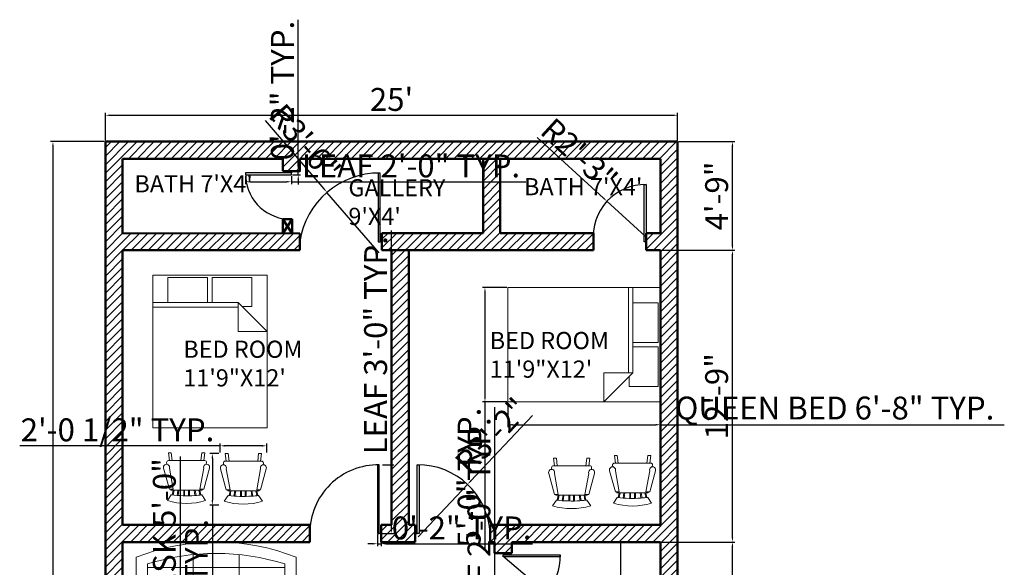
# Model space of a CAD drawing. Units: inches. Extents: x 2308 to 2824, y 1390 to 2024.
# Tile 2 of 2: x 2308 to 2824, y 1737 to 2024. Entities that reach past the tile are written whole.
import ezdxf

# ---------------------------------------------------------------- set-up
doc = ezdxf.new("R2010")
doc.units = ezdxf.units.IN
for name, color, linetype, lineweight in [('A-ANNO-DIMS', 2, 'Continuous', 18), ('A-DOOR', 4, 'Continuous', 25), ('A-FLOR-FIXT', 9, 'Continuous', 25), ('A-FURN', 8, 'Continuous', 18), ('A-WALL', 7, 'Continuous', 50)]:
    doc.layers.add(name, color=color, linetype=linetype, lineweight=lineweight)
doc.layers.add('A-AREA-IDEN', color=244, linetype='Continuous', lineweight=25, true_color=0x991b1e)
doc.layers.add('A-WALL-PATT', color=177, linetype='Continuous', lineweight=13, true_color=0x293189)
doc.styles.get("Standard").update_dxf_attribs({"font": 'arial.ttf'})
doc.dimstyles.new('ISO-25', dxfattribs={"dimtxt": 12, "dimasz": 2.5, "dimexe": 1.25, "dimexo": 0.625, "dimtad": 1, "dimdec": 1, "dimlunit": 3, "dimtxsty": 'Standard', "dimcen": 2.5, "dimadec": 0, "dimazin": 0, "dimtfac": 1, "dimtdec": 1, "dimtmove": 0, "dimatfit": 3, "dimfxl": 1, "dimarcsym": 0})

# ---------------------------------------------------------------- blocks, each defined once
blk = doc.blocks.new('*D1')
at = {"layer": 'A-ANNO-DIMS', "color": 0, "lineweight": -2, "transparency": 16777216}
for p, q in [((2352.46, 1961.09), (2352.46, 1975.53)), ((2354.96, 1974.28), (2649.96, 1974.28)), ((2652.46, 1961.09), (2652.46, 1975.53))]:
    blk.add_line(p, q, dxfattribs=at)
at = {"layer": 'A-ANNO-DIMS', "color": 0, "transparency": 16777216}
for points in [[(2354.96, 1974.7), (2354.96, 1973.86), (2352.46, 1974.28)], [(2649.96, 1974.7), (2649.96, 1973.86), (2652.46, 1974.28)]]:
    blk.add_solid(points, dxfattribs=at)
at = {"layer": 'Defpoints', "color": 0, "transparency": 16777216}
for p in [(2652.46, 1974.28), (2352.46, 1960.47), (2652.46, 1960.47)]:
    blk.add_point(p, dxfattribs=at)
at = {"layer": 'A-ANNO-DIMS', "color": 0, "transparency": 16777216, "insert": (2502.46, 1981.03), "char_height": 12, "attachment_point": 5}
blk.add_mtext("25'", dxfattribs=at)
blk = doc.blocks.new('*D2')
at = {"layer": 'A-ANNO-DIMS', "color": 0, "lineweight": -2, "transparency": 16777216}
for p, q in [((2351.84, 1960.47), (2323.71, 1960.47)), ((2324.96, 1957.97), (2324.96, 1422.97)), ((2351.84, 1420.47), (2323.71, 1420.47))]:
    blk.add_line(p, q, dxfattribs=at)
at = {"layer": 'A-ANNO-DIMS', "color": 0, "transparency": 16777216}
for points in [[(2324.54, 1957.97), (2325.37, 1957.97), (2324.96, 1960.47)], [(2324.54, 1422.97), (2325.37, 1422.97), (2324.96, 1420.47)]]:
    blk.add_solid(points, dxfattribs=at)
at = {"layer": 'Defpoints', "color": 0, "transparency": 16777216}
for p in [(2352.46, 1960.47), (2324.96, 1420.47), (2352.46, 1420.47)]:
    blk.add_point(p, dxfattribs=at)
at = {"layer": 'A-ANNO-DIMS', "color": 0, "transparency": 16777216, "insert": (2318.23, 1690.47), "char_height": 12, "attachment_point": 5, "rotation": 90}
blk.add_mtext("45'", dxfattribs=at)
blk = doc.blocks.new('Bed - Queen')
for p, q in [((0, -80.00003), (0, 0)), ((0, 0), (59.99999, 0)), ((59.99999, 0), (59.99999, -80.00003)), ((7.99999, -1.2), (28.79998, -1.2)), ((7.99999, -14.4), (7.99999, -1.2)), ((28.79998, -1.2), (28.79998, -14.4)), ((31.19999, -1.2), (51.99999, -1.2)), ((31.19999, -14.4), (31.19999, -1.2)), ((51.99999, -1.2), (51.99999, -16.4)), ((0, -14.4), (44.8, -14.4)), ((59.99999, -29.6), (44.8, -14.4)), ((44.8, -14.4), (44.8, -29.6)), ((44.8, -16.8), (0, -16.8)), ((51.99999, -16.4), (46.79936, -16.4)), ((44.8, -29.6), (59.99999, -29.6)), ((59.99999, -80.00003), (0, -80.00003))]:
    blk.add_line(p, q)
blk = doc.blocks.new('Chair - Rocking')
for p, q in [((-8, -4.5), (-10, -1.5)), ((-7.5, -4.5), (-7, -7)), ((-6.5, -7), (-7.02225, -4.43)), ((-4.5, -7), (-4.96674, -4.19951)), ((-4, -7), (-4.40532, -4.16272)), ((-1.5, -4.05012), (-1.5, -7)), ((-1, -7), (-1, -4.05012)), ((1, -7), (1, -4.04655)), ((1.5, -4.05012), (1.5, -7)), ((4, -7), (4.40187, -4.18694)), ((4.5, -7), (4.96761, -4.19437)), ((6.5, -7), (7, -4.4057)), ((7.5, -4.5), (7, -7)), ((8, -4.5), (10, -1.5)), ((-9, -7.5), (-12, -18.49999)), ((-7, -7.5), (-9, -7.5)), ((-9, -18.49999), (-7, -7.5)), ((-8.23428, -6.99939), (-8.3093, -7.47958)), ((-8.23041, -7), (8.23915, -7)), ((7, -7.5), (9, -7.5)), ((9, -18.49999), (7, -7.5)), ((8.31071, -7.48854), (8.23449, -7.00073)), ((9, -7.5), (12, -18.49999)), ((-10.36644, -20.64523), (-10.5, -21.49999)), ((10.5, -21.49999), (10.3575, -20.58798)), ((-9, -22.49999), (-9.5, -26.49999)), ((0, -22.49999), (-9.5, -22.49999)), ((-8, -26.49999), (-7.5, -22.49999)), ((0, -22.49999), (9.5, -22.49999)), ((8, -26.49999), (7.5, -22.49999)), ((9, -22.49999), (9.5, -26.49999)), ((-9.5, -26.49999), (-8, -26.49999)), ((9.5, -26.49999), (8, -26.49999))]:
    blk.add_line(p, q)
for centre, radius, start, end in [((0, -34.08333), 34.08333, 72.93847, 107.0615), ((0, -68.25004), 64.25, 93.92211, 97.15267), ((0, -68.25004), 64.25, 82.84733, 93.92211), ((-10.5, -18.99999), 1.58114, 161.5651, 18.43495), ((10.5, -18.99999), 1.58114, 161.5651, 18.43495), ((-9.5, -21.49999), 1, 180, 270), ((9.5, -21.49999), 1, 270, 0)]:
    blk.add_arc(centre, radius, start, end)
blk = doc.blocks.new('Sofa - Roundback 7 ft.')
for p, q in [((-12.00002, -32.4421), (-12.00003, -6.5971)), ((11.99997, -32.4421), (11.99998, -6.5971)), ((-36.000027, -34), (-36.000027, -11.4696)), ((-35.999844, -13.3819), (35.9998, -13.3819)), ((35.99998, -34), (35.99998, -11.4696)), ((-36.000027, -32.4421), (35.99998, -32.4421))]:
    blk.add_line(p, q)
for points in [[(-36.000027, -34), (-42.000027, -34), (-42.000027, -8)], [(41.99998, -8), (41.99998, -34), (35.99998, -34)]]:
    blk.add_lwpolyline(points)
for centre, radius, start, end in [((0, -114.25), 114.25, 68.43141, 111.5686), ((-0.00001, -127.1968), 121.1968, 72.72033, 107.2797)]:
    blk.add_arc(centre, radius, start, end)
blk = doc.blocks.new('DOOR-LEAF-36IN')
for p, q in [((-1, 36), (-2, 36)), ((-2, 36), (-2, 0)), ((-1, 0), (-1, 36)), ((-2, 0), (-1, 0)), ((0, 0), (-1, 0))]:
    blk.add_line(p, q)
blk = doc.blocks.new('DOOR-LEAF-24IN')
for p, q in [((0, 0), (0, -1)), ((0, -1), (-24, -1)), ((-24, -1), (-24, -2)), ((-24, -2), (0, -2)), ((0, -2), (0, -1))]:
    blk.add_line(p, q)
blk = doc.blocks.new('*D11')
at = {"layer": 'A-ANNO-DIMS', "color": 0, "lineweight": -2, "transparency": 16777216}
for p, q in [((2411.97, 1796.88), (2407.29, 1796.88)), ((2408.54, 1794.38), (2408.54, 1772.38)), ((2411.97, 1769.88), (2407.29, 1769.88)), ((2408.54, 1769.88), (2408.54, 1617.23))]:
    blk.add_line(p, q, dxfattribs=at)
at = {"layer": 'A-ANNO-DIMS', "color": 0, "transparency": 16777216}
for points in [[(2408.13, 1794.38), (2408.96, 1794.38), (2408.54, 1796.88)], [(2408.13, 1772.38), (2408.96, 1772.38), (2408.54, 1769.88)]]:
    blk.add_solid(points, dxfattribs=at)
at = {"layer": 'Defpoints', "color": 0, "transparency": 16777216}
for p in [(2412.59, 1796.88), (2408.54, 1769.88), (2412.59, 1769.88)]:
    blk.add_point(p, dxfattribs=at)
at = {"layer": 'A-ANNO-DIMS', "color": 0, "transparency": 16777216, "insert": (2401.7, 1692.31), "char_height": 12, "attachment_point": 5, "rotation": 90}
blk.add_mtext('ROCKER 2\'-3" TYP.', dxfattribs=at)
blk = doc.blocks.new('*D12')
at = {"layer": 'A-ANNO-DIMS', "color": 0, "lineweight": -2, "transparency": 16777216}
for p, q in [((2412.59, 1797.51), (2412.59, 1802.18)), ((2437.03, 1797.51), (2437.03, 1802.18)), ((2412.59, 1800.93), (2307.53, 1800.93)), ((2434.53, 1800.93), (2415.09, 1800.93))]:
    blk.add_line(p, q, dxfattribs=at)
at = {"layer": 'A-ANNO-DIMS', "color": 0, "transparency": 16777216}
for points in [[(2415.09, 1801.35), (2415.09, 1800.52), (2412.59, 1800.93)], [(2434.53, 1801.35), (2434.53, 1800.52), (2437.03, 1800.93)]]:
    blk.add_solid(points, dxfattribs=at)
at = {"layer": 'Defpoints', "color": 0, "transparency": 16777216}
for p in [(2412.59, 1800.93), (2412.59, 1796.88), (2437.03, 1796.88)]:
    blk.add_point(p, dxfattribs=at)
at = {"layer": 'A-ANNO-DIMS', "color": 0, "transparency": 16777216, "insert": (2358.81, 1807.76), "char_height": 12, "attachment_point": 5}
blk.add_mtext('2\'-0 1/2" TYP.', dxfattribs=at)
blk = doc.blocks.new('*D15')
at = {"layer": 'A-ANNO-DIMS', "color": 0, "lineweight": -2, "transparency": 16777216}
for p, q in [((2563.46, 1823.36), (2563.46, 1810.73)), ((2643.46, 1823.36), (2643.46, 1810.73)), ((2565.96, 1811.98), (2640.96, 1811.98)), ((2643.46, 1811.98), (2823.73, 1811.98))]:
    blk.add_line(p, q, dxfattribs=at)
at = {"layer": 'A-ANNO-DIMS', "color": 0, "transparency": 16777216}
for points in [[(2565.96, 1812.4), (2565.96, 1811.56), (2563.46, 1811.98)], [(2640.96, 1812.4), (2640.96, 1811.56), (2643.46, 1811.98)]]:
    blk.add_solid(points, dxfattribs=at)
at = {"layer": 'Defpoints', "color": 0, "transparency": 16777216}
for p in [(2563.46, 1823.98), (2643.46, 1823.98), (2643.46, 1811.98)]:
    blk.add_point(p, dxfattribs=at)
at = {"layer": 'A-ANNO-DIMS', "color": 0, "transparency": 16777216, "insert": (2734.85, 1819.18), "char_height": 12, "attachment_point": 5}
blk.add_mtext('QUEEN BED 6\'-8" TYP.', dxfattribs=at)
blk = doc.blocks.new('*D16')
at = {"layer": 'A-ANNO-DIMS', "color": 0, "lineweight": -2, "transparency": 16777216}
for p, q in [((2562.84, 1883.98), (2550.21, 1883.98)), ((2551.46, 1881.48), (2551.46, 1826.48)), ((2562.84, 1823.98), (2550.21, 1823.98)), ((2551.46, 1823.98), (2551.46, 1747.09))]:
    blk.add_line(p, q, dxfattribs=at)
at = {"layer": 'A-ANNO-DIMS', "color": 0, "transparency": 16777216}
for points in [[(2551.04, 1881.48), (2551.88, 1881.48), (2551.46, 1883.98)], [(2551.04, 1826.48), (2551.88, 1826.48), (2551.46, 1823.98)]]:
    blk.add_solid(points, dxfattribs=at)
at = {"layer": 'Defpoints', "color": 0, "transparency": 16777216}
for p in [(2563.46, 1883.98), (2551.46, 1823.98), (2563.46, 1823.98)]:
    blk.add_point(p, dxfattribs=at)
at = {"layer": 'A-ANNO-DIMS', "color": 0, "transparency": 16777216, "insert": (2544.71, 1784.28), "char_height": 12, "attachment_point": 5, "rotation": 90}
blk.add_mtext('5\'-0" TYP.', dxfattribs=at)
blk = doc.blocks.new('*D17')
at = {"layer": 'A-ANNO-DIMS', "color": 0, "lineweight": -2, "transparency": 16777216}
for p, q in [((2391.75, 1710.04), (2391.75, 1795.4)), ((2400.13, 1710.04), (2390.5, 1710.04)), ((2391.75, 1652.54), (2391.75, 1707.54)), ((2400.13, 1650.04), (2390.5, 1650.04))]:
    blk.add_line(p, q, dxfattribs=at)
at = {"layer": 'A-ANNO-DIMS', "color": 0, "transparency": 16777216}
for points in [[(2391.34, 1707.54), (2392.17, 1707.54), (2391.75, 1710.04)], [(2391.34, 1652.54), (2392.17, 1652.54), (2391.75, 1650.04)]]:
    blk.add_solid(points, dxfattribs=at)
at = {"layer": 'Defpoints', "color": 0, "transparency": 16777216}
for p in [(2391.75, 1710.04), (2400.75, 1710.04), (2400.75, 1650.04)]:
    blk.add_point(p, dxfattribs=at)
at = {"layer": 'A-ANNO-DIMS', "color": 0, "transparency": 16777216, "insert": (2384.92, 1753.97), "char_height": 12, "attachment_point": 5, "rotation": 90}
blk.add_mtext('DESK 5\'-0"', dxfattribs=at)
blk = doc.blocks.new('*D19')
at = {"layer": 'A-ANNO-DIMS', "color": 0, "lineweight": -2, "transparency": 16777216}
for p, q in [((2502.44, 1790.97), (2502.44, 1913.91)), ((2497.66, 1790.97), (2503.69, 1790.97)), ((2502.44, 1757.47), (2502.44, 1788.47)), ((2497.66, 1754.97), (2503.69, 1754.97))]:
    blk.add_line(p, q, dxfattribs=at)
at = {"layer": 'A-ANNO-DIMS', "color": 0, "transparency": 16777216}
for points in [[(2502.02, 1788.47), (2502.85, 1788.47), (2502.44, 1790.97)], [(2502.02, 1757.47), (2502.85, 1757.47), (2502.44, 1754.97)]]:
    blk.add_solid(points, dxfattribs=at)
at = {"layer": 'Defpoints', "color": 0, "transparency": 16777216}
for p in [(2497.04, 1790.97), (2502.44, 1790.97), (2497.04, 1754.97)]:
    blk.add_point(p, dxfattribs=at)
at = {"layer": 'A-ANNO-DIMS', "color": 0, "transparency": 16777216, "insert": (2495.68, 1853.69), "char_height": 12, "attachment_point": 5, "rotation": 90}
blk.add_mtext('LEAF 3\'-0" TYP.', dxfattribs=at)
blk = doc.blocks.new('*D20')
at = {"layer": 'A-ANNO-DIMS', "color": 0, "lineweight": -2, "transparency": 16777216}
for p, q in [((2495.04, 1754.34), (2495.04, 1748.32)), ((2497.04, 1754.34), (2497.04, 1748.32)), ((2492.54, 1749.57), (2490.04, 1749.57)), ((2495.04, 1749.57), (2497.04, 1749.57)), ((2499.54, 1749.57), (2576.43, 1749.57))]:
    blk.add_line(p, q, dxfattribs=at)
at = {"layer": 'A-ANNO-DIMS', "color": 0, "transparency": 16777216}
for points in [[(2492.54, 1749.98), (2492.54, 1749.15), (2495.04, 1749.57)], [(2499.54, 1749.98), (2499.54, 1749.15), (2497.04, 1749.57)]]:
    blk.add_solid(points, dxfattribs=at)
at = {"layer": 'Defpoints', "color": 0, "transparency": 16777216}
for p in [(2495.04, 1754.97), (2497.04, 1754.97), (2497.04, 1749.57)]:
    blk.add_point(p, dxfattribs=at)
at = {"layer": 'A-ANNO-DIMS', "color": 0, "transparency": 16777216, "insert": (2539.23, 1756.32), "char_height": 12, "attachment_point": 5}
blk.add_mtext('0\'-2" TYP.', dxfattribs=at)
blk = doc.blocks.new('*D21')
at = {"layer": 'A-ANNO-DIMS', "color": 0, "lineweight": -2, "transparency": 16777216}
for p, q in [((2425.96, 1942.39), (2425.96, 1938.16)), ((2449.96, 1942.39), (2449.96, 1938.16)), ((2428.46, 1939.41), (2447.46, 1939.41)), ((2449.96, 1939.41), (2572.91, 1939.41))]:
    blk.add_line(p, q, dxfattribs=at)
at = {"layer": 'A-ANNO-DIMS', "color": 0, "transparency": 16777216}
for points in [[(2428.46, 1939.83), (2428.46, 1939), (2425.96, 1939.41)], [(2447.46, 1939.83), (2447.46, 1939), (2449.96, 1939.41)]]:
    blk.add_solid(points, dxfattribs=at)
at = {"layer": 'Defpoints', "color": 0, "transparency": 16777216}
for p in [(2425.96, 1943.01), (2449.96, 1943.01), (2449.96, 1939.41)]:
    blk.add_point(p, dxfattribs=at)
at = {"layer": 'A-ANNO-DIMS', "color": 0, "transparency": 16777216, "insert": (2512.68, 1946.17), "char_height": 12, "attachment_point": 5}
blk.add_mtext('LEAF 2\'-0" TYP.', dxfattribs=at)
blk = doc.blocks.new('*D22')
at = {"layer": 'A-ANNO-DIMS', "color": 0, "lineweight": -2, "transparency": 16777216}
for p, q in [((2453.56, 1947.51), (2453.56, 2024.41)), ((2450.59, 1945.01), (2454.81, 1945.01)), ((2450.59, 1943.01), (2454.81, 1943.01)), ((2453.56, 1943.01), (2453.56, 1945.01)), ((2453.56, 1940.51), (2453.56, 1938.01))]:
    blk.add_line(p, q, dxfattribs=at)
at = {"layer": 'A-ANNO-DIMS', "color": 0, "transparency": 16777216}
for points in [[(2453.14, 1947.51), (2453.98, 1947.51), (2453.56, 1945.01)], [(2453.14, 1940.51), (2453.98, 1940.51), (2453.56, 1943.01)]]:
    blk.add_solid(points, dxfattribs=at)
at = {"layer": 'Defpoints', "color": 0, "transparency": 16777216}
for p in [(2449.96, 1945.01), (2449.96, 1943.01), (2453.56, 1945.01)]:
    blk.add_point(p, dxfattribs=at)
at = {"layer": 'A-ANNO-DIMS', "color": 0, "transparency": 16777216, "insert": (2446.81, 1987.21), "char_height": 12, "attachment_point": 5, "rotation": 90}
blk.add_mtext('0\'-2" TYP.', dxfattribs=at)
blk = doc.blocks.new('*D23')
at = {"layer": 'A-ANNO-DIMS', "color": 0, "lineweight": -2, "transparency": 16777216}
for p, q in [((2556.62, 1654.47), (2556.62, 1821.13)), ((2553.65, 1654.47), (2557.87, 1654.47)), ((2556.62, 1632.97), (2556.62, 1651.97)), ((2553.65, 1630.47), (2557.87, 1630.47))]:
    blk.add_line(p, q, dxfattribs=at)
at = {"layer": 'A-ANNO-DIMS', "color": 0, "transparency": 16777216}
for points in [[(2556.21, 1651.97), (2557.04, 1651.97), (2556.62, 1654.47)], [(2556.21, 1632.97), (2557.04, 1632.97), (2556.62, 1630.47)]]:
    blk.add_solid(points, dxfattribs=at)
at = {"layer": 'Defpoints', "color": 0, "transparency": 16777216}
for p in [(2553.02, 1654.47), (2556.62, 1654.47), (2553.02, 1630.47)]:
    blk.add_point(p, dxfattribs=at)
at = {"layer": 'A-ANNO-DIMS', "color": 0, "transparency": 16777216, "insert": (2549.87, 1739.05), "char_height": 12, "attachment_point": 5, "rotation": 90}
blk.add_mtext('PAIR LEAF 2\'-0" TYP.', dxfattribs=at)
blk = doc.blocks.new('*D33')
at = {"layer": 'A-ANNO-DIMS', "color": 0, "lineweight": -2, "transparency": 16777216}
for p, q in [((2644.09, 1750.47), (2682.46, 1750.47)), ((2681.21, 1632.97), (2681.21, 1747.97)), ((2644.09, 1630.47), (2682.46, 1630.47))]:
    blk.add_line(p, q, dxfattribs=at)
at = {"layer": 'A-ANNO-DIMS', "color": 0, "transparency": 16777216}
for points in [[(2680.79, 1747.97), (2681.63, 1747.97), (2681.21, 1750.47)], [(2680.79, 1632.97), (2681.63, 1632.97), (2681.21, 1630.47)]]:
    blk.add_solid(points, dxfattribs=at)
at = {"layer": 'Defpoints', "color": 0, "transparency": 16777216}
for p in [(2643.46, 1750.47), (2681.21, 1750.47), (2643.46, 1630.47)]:
    blk.add_point(p, dxfattribs=at)
at = {"layer": 'A-ANNO-DIMS', "color": 0, "transparency": 16777216, "insert": (2674.46, 1690.47), "char_height": 12, "attachment_point": 5, "rotation": 90}
blk.add_mtext('10\'-0"', dxfattribs=at)
blk = doc.blocks.new('*D34')
at = {"layer": 'A-ANNO-DIMS', "color": 0, "lineweight": -2, "transparency": 16777216}
for p, q in [((2644.09, 1903.47), (2682.46, 1903.47)), ((2681.21, 1752.97), (2681.21, 1900.97)), ((2644.09, 1750.47), (2682.46, 1750.47))]:
    blk.add_line(p, q, dxfattribs=at)
at = {"layer": 'A-ANNO-DIMS', "color": 0, "transparency": 16777216}
for points in [[(2680.79, 1900.97), (2681.63, 1900.97), (2681.21, 1903.47)], [(2680.79, 1752.97), (2681.63, 1752.97), (2681.21, 1750.47)]]:
    blk.add_solid(points, dxfattribs=at)
at = {"layer": 'Defpoints', "color": 0, "transparency": 16777216}
for p in [(2643.46, 1903.47), (2681.21, 1903.47), (2643.46, 1750.47)]:
    blk.add_point(p, dxfattribs=at)
at = {"layer": 'A-ANNO-DIMS', "color": 0, "transparency": 16777216, "insert": (2674.46, 1826.97), "char_height": 12, "attachment_point": 5, "rotation": 90}
blk.add_mtext('12\'-9"', dxfattribs=at)
blk = doc.blocks.new('*D35')
at = {"layer": 'A-ANNO-DIMS', "color": 0, "lineweight": -2, "transparency": 16777216}
for p, q in [((2653.09, 1960.47), (2682.46, 1960.47)), ((2681.21, 1905.97), (2681.21, 1957.97)), ((2644.09, 1903.47), (2682.46, 1903.47))]:
    blk.add_line(p, q, dxfattribs=at)
at = {"layer": 'A-ANNO-DIMS', "color": 0, "transparency": 16777216}
for points in [[(2680.79, 1957.97), (2681.63, 1957.97), (2681.21, 1960.47)], [(2680.79, 1905.97), (2681.63, 1905.97), (2681.21, 1903.47)]]:
    blk.add_solid(points, dxfattribs=at)
at = {"layer": 'Defpoints', "color": 0, "transparency": 16777216}
for p in [(2652.46, 1960.47), (2681.21, 1960.47), (2643.46, 1903.47)]:
    blk.add_point(p, dxfattribs=at)
at = {"layer": 'A-ANNO-DIMS', "color": 0, "transparency": 16777216, "insert": (2674.46, 1931.97), "char_height": 12, "attachment_point": 5, "rotation": 90}
blk.add_mtext('4\'-9"', dxfattribs=at)
blk = doc.blocks.new('*D37')
at = {"layer": 'A-ANNO-DIMS', "color": 0, "lineweight": -2, "transparency": 16777216}
for p, q in [((2436.25, 1971.46), (2466.99, 1935.73)), ((2495.93, 1902.1), (2468.62, 1933.84))]:
    blk.add_line(p, q, dxfattribs=at)
at = {"layer": 'A-ANNO-DIMS', "color": 0, "transparency": 16777216}
blk.add_solid([(2467.31, 1936.01), (2466.68, 1935.46), (2468.62, 1933.84)], dxfattribs=at)
at = {"layer": 'Defpoints', "color": 0, "transparency": 16777216}
for p in [(2468.62, 1933.84), (2495.93, 1902.1)]:
    blk.add_point(p, dxfattribs=at)
at = {"layer": 'A-ANNO-DIMS', "color": 0, "transparency": 16777216, "insert": (2455.93, 1958.95), "char_height": 12, "attachment_point": 5, "rotation": 310.7086}
blk.add_mtext('R3\'-6"', dxfattribs=at)
blk = doc.blocks.new('*D38')
at = {"layer": 'A-ANNO-DIMS', "color": 0, "lineweight": -2, "transparency": 16777216}
for p, q in [((2576.32, 1816.83), (2544.02, 1782.52)), ((2516.4, 1753.19), (2542.3, 1780.7))]:
    blk.add_line(p, q, dxfattribs=at)
at = {"layer": 'A-ANNO-DIMS', "color": 0, "transparency": 16777216}
blk.add_solid([(2543.71, 1782.8), (2544.32, 1782.23), (2542.3, 1780.7)], dxfattribs=at)
at = {"layer": 'Defpoints', "color": 0, "transparency": 16777216}
for p in [(2542.3, 1780.7), (2516.4, 1753.19)]:
    blk.add_point(p, dxfattribs=at)
at = {"layer": 'A-ANNO-DIMS', "color": 0, "transparency": 16777216, "insert": (2556.11, 1805.22), "char_height": 12, "attachment_point": 5, "rotation": 46.7258}
blk.add_mtext('R3\'-2"', dxfattribs=at)
blk = doc.blocks.new('*D39')
at = {"layer": 'A-ANNO-DIMS', "color": 0, "lineweight": -2, "transparency": 16777216}
for p, q in [((2560.86, 1743.18), (2583.88, 1723.78)), ((2621.83, 1691.79), (2585.79, 1722.17))]:
    blk.add_line(p, q, dxfattribs=at)
at = {"layer": 'A-ANNO-DIMS', "color": 0, "transparency": 16777216}
blk.add_solid([(2586.06, 1722.48), (2585.52, 1721.85), (2583.88, 1723.78)], dxfattribs=at)
at = {"layer": 'Defpoints', "color": 0, "transparency": 16777216}
for p in [(2560.86, 1743.18), (2583.88, 1723.78)]:
    blk.add_point(p, dxfattribs=at)
at = {"layer": 'A-ANNO-DIMS', "color": 0, "transparency": 16777216, "insert": (2609.12, 1711.33), "char_height": 12, "attachment_point": 5, "rotation": 319.8697}
blk.add_mtext('R2\'-6"', dxfattribs=at)
blk = doc.blocks.new('*D40')
at = {"layer": 'A-ANNO-DIMS', "color": 0, "lineweight": -2, "transparency": 16777216}
for p, q in [((2578.82, 1962.69), (2613.57, 1930.85)), ((2635.42, 1910.84), (2615.42, 1929.17))]:
    blk.add_line(p, q, dxfattribs=at)
at = {"layer": 'A-ANNO-DIMS', "color": 0, "transparency": 16777216}
blk.add_solid([(2613.85, 1931.16), (2613.29, 1930.55), (2615.42, 1929.17)], dxfattribs=at)
at = {"layer": 'Defpoints', "color": 0, "transparency": 16777216}
for p in [(2615.42, 1929.17), (2635.42, 1910.84)]:
    blk.add_point(p, dxfattribs=at)
at = {"layer": 'A-ANNO-DIMS', "color": 0, "transparency": 16777216, "insert": (2599.84, 1952.6), "char_height": 12, "attachment_point": 5, "rotation": 317.5117}
blk.add_mtext('R2\'-3"', dxfattribs=at)

msp = doc.modelspace()

# ---------------------------------------------------------------- hatches: boundary and pattern name
at = {"layer": 'A-WALL-PATT'}
h = msp.add_hatch(dxfattribs=at)
h.set_pattern_fill('ANSI31', color=256)
h.paths.add_polyline_path([(2361.46, 1750.47), (2459.65, 1750.47), (2459.65, 1759.47), (2361.46, 1759.47), (2361.46, 1903.47), (2454.46, 1903.47), (2454.46, 1912.24), (2361.46, 1912.47), (2361.46, 1951.47), (2445.46, 1951.47), (2445.46, 1945.01), (2454.46, 1945.01), (2454.46, 1951.47), (2643.46, 1951.47), (2643.46, 1912.47), (2635.92, 1912.47), (2635.92, 1903.47), (2643.46, 1903.47), (2643.46, 1759.47), (2554.14, 1759.47), (2554.14, 1750.47), (2556.46, 1750.47), (2556.46, 1744.68), (2565.46, 1744.68), (2565.46, 1750.47), (2643.46, 1750.47), (2643.46, 1639.47), (2565.46, 1639.47), (2565.46, 1713.43), (2556.46, 1713.43), (2556.46, 1639.47), (2553.02, 1639.47), (2553.02, 1630.47), (2643.46, 1630.47), (2643.46, 1429.47), (2643.46, 1420.47), (2652.46, 1420.47), (2652.46, 1960.47), (2352.46, 1960.47), (2352.46, 1420.47), (2505.46, 1420.47), (2505.46, 1429.47), (2430.46, 1429.47), (2430.46, 1439.34), (2421.46, 1439.34), (2421.46, 1429.47), (2361.46, 1429.47), (2361.46, 1468.47), (2421.46, 1468.47), (2421.46, 1465.33), (2430.46, 1465.33), (2430.46, 1468.47), (2505.46, 1468.47), (2505.46, 1477.47), (2505.46, 1486.65), (2496.46, 1486.65), (2496.46, 1477.47), (2361.46, 1477.47), (2361.46, 1630.47), (2496.46, 1630.47), (2496.46, 1533.54), (2505.46, 1533.54), (2505.46, 1630.47), (2505.46, 1639.47), (2503.24, 1639.47), (2361.46, 1639.47)])
h.paths.add_polyline_path([(2511.46, 1903.47), (2502.46, 1903.47), (2502.46, 1759.47), (2497.04, 1759.47), (2497.04, 1750.47), (2514.9, 1750.47), (2514.9, 1759.47), (2511.46, 1759.47)], flags=17)
h.paths.add_polyline_path([(2608.34, 1912.47), (2559.46, 1912.47), (2559.46, 1951.47), (2550.46, 1951.47), (2550.46, 1912.47), (2497.43, 1912.47), (2497.43, 1903.47), (2608.44, 1903.47), (2608.44, 1907.97, -0.041548)], flags=17)
h.paths.add_polyline_path([(2360.24, 1427.17), (2428.94, 1427.17), (2428.94, 1445.72), (2360.24, 1445.72)], flags=24)

# ---------------------------------------------------------------- linework, layer by layer
at = {"layer": 'A-DOOR'}
for p, q in [((2634.92, 1907.97), (2634.92, 1937.97)), ((2634.92, 1937.97), (2635.92, 1937.97)), ((2635.92, 1937.97), (2635.92, 1912.47)), ((2635.92, 1907.97), (2634.92, 1907.97)), ((2560.96, 1744.68), (2560.96, 1743.68)), ((2560.96, 1743.68), (2590.96, 1743.68)), ((2560.96, 1742.68), (2560.96, 1743.68)), ((2590.96, 1742.68), (2560.96, 1742.68)), ((2590.96, 1743.68), (2590.96, 1742.68))]:
    msp.add_line(p, q, dxfattribs=at)
for centre, radius, start, end in [((2449.79, 1943.51), 23.83, 178.7979, 265.4489), ((2495.93, 1902.1), 41.87, 89.3158, 172.102), ((2635.42, 1910.84), 27.13, 88.944, 186.0803), ((2495.54, 1755.08), 35.89, 89.2017, 180.186), ((2516.4, 1753.19), 37.78, 2.6938, 90.7583), ((2560.86, 1743.18), 30.1, 278.7856, 0.9517)]:
    msp.add_arc(centre, radius, start, end, dxfattribs=at)
at = {"layer": 'A-FLOR-FIXT'}
msp.add_line((2622.77, 1661.84), (2622.77, 1750.47), dxfattribs=at)
at = {"layer": 'A-WALL'}
for p, q in [((2352.46, 1960.47), (2652.46, 1960.47)), ((2352.46, 1420.47), (2352.46, 1960.47)), ((2652.46, 1960.47), (2652.46, 1420.47)), ((2361.46, 1951.47), (2445.46, 1951.47)), ((2361.46, 1912.47), (2361.46, 1951.47)), ((2445.46, 1945.01), (2445.46, 1951.47)), ((2454.46, 1945.01), (2454.46, 1951.47)), ((2454.46, 1951.47), (2643.46, 1951.47)), ((2550.46, 1951.47), (2550.46, 1912.47)), ((2559.46, 1951.47), (2559.46, 1912.47)), ((2643.46, 1951.47), (2643.46, 1912.47)), ((2445.46, 1945.01), (2454.46, 1945.01)), ((2445.46, 1912.26), (2445.46, 1919.76)), ((2445.46, 1919.76), (2450.33, 1919.76)), ((2450.32, 1912.25), (2445.46, 1919.76)), ((2445.46, 1912.26), (2450.33, 1919.76)), ((2450.33, 1919.76), (2450.32, 1912.25)), ((2361.46, 1912.47), (2454.46, 1912.24)), ((2454.46, 1903.47), (2454.46, 1912.24)), ((2497.43, 1912.47), (2550.46, 1912.47)), ((2497.43, 1912.47), (2497.43, 1903.47)), ((2559.46, 1912.47), (2608.44, 1912.47)), ((2608.44, 1912.47), (2608.44, 1903.47)), ((2635.92, 1912.47), (2635.92, 1903.47)), ((2635.92, 1912.47), (2643.46, 1912.47)), ((2361.46, 1903.47), (2454.46, 1903.47)), ((2361.46, 1759.47), (2361.46, 1903.47)), ((2497.43, 1903.47), (2608.44, 1903.47)), ((2502.46, 1759.47), (2502.46, 1903.47)), ((2511.46, 1759.47), (2511.46, 1903.47)), ((2635.92, 1903.47), (2643.46, 1903.47)), ((2643.46, 1903.47), (2643.46, 1759.47)), ((2361.46, 1759.47), (2459.65, 1759.47)), ((2459.65, 1759.47), (2459.65, 1750.47)), ((2497.04, 1759.47), (2497.04, 1750.47)), ((2497.04, 1759.47), (2502.46, 1759.47)), ((2511.46, 1759.47), (2514.9, 1759.47)), ((2514.9, 1759.47), (2514.9, 1750.47)), ((2554.14, 1759.47), (2554.14, 1750.47)), ((2554.14, 1759.47), (2643.46, 1759.47)), ((2361.46, 1750.47), (2459.65, 1750.47)), ((2361.46, 1639.47), (2361.46, 1750.47)), ((2497.04, 1750.47), (2514.9, 1750.47)), ((2554.14, 1750.47), (2556.46, 1750.47)), ((2556.46, 1750.47), (2556.46, 1744.68)), ((2565.46, 1750.47), (2565.46, 1744.68)), ((2565.46, 1750.47), (2643.46, 1750.47)), ((2643.46, 1750.47), (2643.46, 1639.47)), ((2565.46, 1744.68), (2556.46, 1744.68))]:
    msp.add_line(p, q, dxfattribs=at)

# ---------------------------------------------------------------- block references
at = {"layer": 'A-DOOR'}
for name, p in [('DOOR-LEAF-24IN', (2449.96, 1945.01)), ('DOOR-LEAF-36IN', (2497.43, 1907.97)), ('DOOR-LEAF-36IN', (2497.04, 1754.97))]:
    msp.add_blockref(name, p, dxfattribs=at)
at = {"layer": 'A-DOOR', "extrusion": (0, 0, -1), "zscale": -1}
msp.add_blockref('DOOR-LEAF-36IN', (-2514.9, 1754.97), dxfattribs=at)
at = {"layer": 'A-FURN'}
for name, p in [('Bed - Queen', (2377.25, 1890.41)), ('Sofa - Roundback 7 ft.', (2410.55, 1750.47))]:
    msp.add_blockref(name, p, dxfattribs=at)
for name, p, rotation in [('Bed - Queen', (2643.46, 1883.98), 270), ('Chair - Rocking', (2395.01, 1770.71), 180), ('Chair - Rocking', (2424.81, 1770.38), 180), ('Chair - Rocking', (2596.88, 1767.97), 180), ('Chair - Rocking', (2628.83, 1769.35), 180)]:
    msp.add_blockref(name, p, dxfattribs=dict(at, rotation=rotation))

# ---------------------------------------------------------------- texts
at = {"layer": 'A-AREA-IDEN', "char_height": 9, "attachment_point": 1}
for s, width, insert in [("BATH 7'X4'", 64.432, (2367.68, 1942.85)), ("GALLERY\\P9'X4'", 64.432, (2479.87, 1940.77)), ("BATH 7'X4'", 64.432, (2571.93, 1941.32)), ('BED ROOM\\P11\'9"X12\'', 73.3205, (2553.97, 1860.65)), ('BED ROOM\\P11\'9"X12\'', 80.6383, (2393.32, 1856.08))]:
    msp.add_mtext_dynamic_manual_height_columns(s, width=width, gutter_width=12.5, heights=[0], dxfattribs=dict(at, insert=insert))

# ---------------------------------------------------------------- dimensions: what is measured, and where the dimension line sits
at = {"layer": 'A-ANNO-DIMS'}
for base, p1, p2, angle, text, picture, middle in [((2453.56, 1945.01), (2449.96, 1943.01), (2449.96, 1945.01), 90, '<> TYP.', '*D22', (2446.81, 1987.21)), ((2502.44, 1790.97), (2497.04, 1754.97), (2497.04, 1790.97), 90, 'LEAF <> TYP.', '*D19', (2495.68, 1853.69)), ((2551.46, 1823.98), (2563.46, 1883.98), (2563.46, 1823.98), 270, '<> TYP.', '*D16', (2544.71, 1784.28)), ((2412.59, 1800.93), (2437.03, 1796.88), (2412.59, 1796.88), 180, '<> TYP.', '*D12', (2358.81, 1807.76)), ((2556.62, 1654.47), (2553.02, 1630.47), (2553.02, 1654.47), 90, 'PAIR LEAF <> TYP.', '*D23', (2549.87, 1739.05)), ((2408.54, 1769.88), (2412.59, 1796.88), (2412.59, 1769.88), 270, 'ROCKER <> TYP.', '*D11', (2401.7, 1692.31)), ((2391.75, 1710.04), (2400.75, 1650.04), (2400.75, 1710.04), 90, 'DESK <>', '*D17', (2384.92, 1753.97))]:
    dim = msp.add_linear_dim(base=base, p1=p1, p2=p2, angle=angle, text=text, dimstyle='ISO-25', override={"dimdec": 1, "dimlfac": 1, "dimrnd": 0, "dimzin": 1, "dimdsep": 46, "dimlunit": 4, "dimfrac": 2}, dxfattribs=at)
    dim.commit()
    dim.dimension.update_dxf_attribs({"geometry": picture, "text_midpoint": middle})
dim = msp.add_linear_dim(base=(2652.46, 1974.28), p1=(2352.46, 1960.47), p2=(2652.46, 1960.47), dimstyle='ISO-25', override={"dimclrd": 0, "dimclre": 0, "dimclrt": 0}, dxfattribs=at)
dim.commit()
dim.dimension.update_dxf_attribs({"geometry": '*D1', "text_midpoint": (2502.46, 1981.03)})
for center, mpoint, picture, middle in [((2495.93, 1902.1), (2468.62, 1933.84), '*D37', (2455.93, 1958.95)), ((2635.42, 1910.84), (2615.42, 1929.17), '*D40', (2599.84, 1952.6)), ((2516.4, 1753.19), (2542.3, 1780.7), '*D38', (2556.11, 1805.22)), ((2560.86, 1743.18), (2583.88, 1723.78), '*D39', (2609.12, 1711.33))]:
    dim = msp.add_radius_dim(center=center, mpoint=mpoint, dimstyle='ISO-25', override={"dimdec": 1, "dimlfac": 1, "dimrnd": 0, "dimzin": 1, "dimdsep": 46, "dimlunit": 4, "dimfrac": 2}, dxfattribs=at)
    dim.commit()
    dim.dimension.update_dxf_attribs({"geometry": picture, "text_midpoint": middle})
for base, p1, p2, text, picture, middle in [((2449.96, 1939.41), (2425.96, 1943.01), (2449.96, 1943.01), 'LEAF <> TYP.', '*D21', (2512.68, 1946.17)), ((2643.46, 1811.98), (2563.46, 1823.98), (2643.46, 1823.98), 'QUEEN BED <> TYP.', '*D15', (2734.85, 1819.18)), ((2497.04, 1749.57), (2495.04, 1754.97), (2497.04, 1754.97), '<> TYP.', '*D20', (2539.23, 1756.32))]:
    dim = msp.add_linear_dim(base=base, p1=p1, p2=p2, text=text, dimstyle='ISO-25', override={"dimdec": 1, "dimlfac": 1, "dimrnd": 0, "dimzin": 1, "dimdsep": 46, "dimlunit": 4, "dimfrac": 2}, dxfattribs=at)
    dim.commit()
    dim.dimension.update_dxf_attribs({"geometry": picture, "text_midpoint": middle})
for base, p1, p2, override, picture, middle in [((2324.96, 1420.47), (2352.46, 1960.47), (2352.46, 1420.47), {"dimclrd": 0, "dimclre": 0, "dimclrt": 0}, '*D2', (2318.23, 1690.47)), ((2681.21, 1960.47), (2643.46, 1903.47), (2652.46, 1960.47), {"dimdec": 1, "dimlfac": 1, "dimrnd": 0, "dimzin": 1, "dimdsep": 46, "dimlunit": 4, "dimfrac": 2}, '*D35', (2674.46, 1931.97)), ((2681.21, 1903.47), (2643.46, 1750.47), (2643.46, 1903.47), {"dimdec": 1, "dimlfac": 1, "dimrnd": 0, "dimzin": 1, "dimdsep": 46, "dimlunit": 4, "dimfrac": 2}, '*D34', (2674.46, 1826.97)), ((2681.21, 1750.47), (2643.46, 1630.47), (2643.46, 1750.47), {"dimdec": 1, "dimlfac": 1, "dimrnd": 0, "dimzin": 1, "dimdsep": 46, "dimlunit": 4, "dimfrac": 2}, '*D33', (2674.46, 1690.47))]:
    dim = msp.add_linear_dim(base=base, p1=p1, p2=p2, angle=90, dimstyle='ISO-25', override=override, dxfattribs=at)
    dim.commit()
    dim.dimension.update_dxf_attribs({"geometry": picture, "text_midpoint": middle})

doc.saveas('drawing.dxf')
